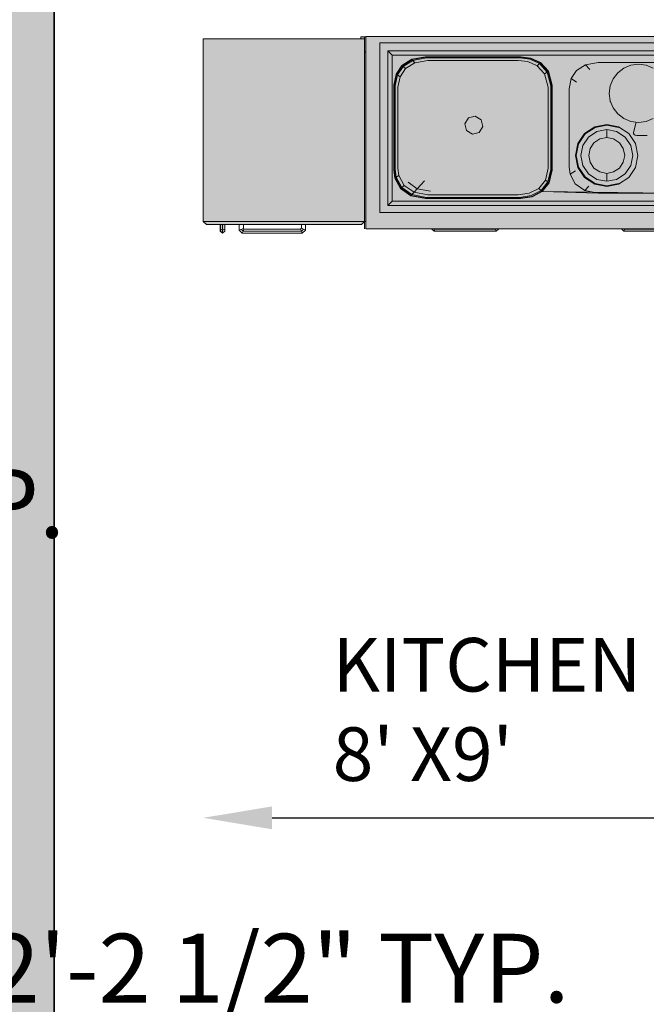
# Model space of a CAD drawing. Units: inches. Extents: x 2178 to 3409, y 1711 to 2279.
# Tile 5 of 8: x 2368 to 2423, y 2140 to 2226. Entities that reach past the tile are written whole.
import ezdxf

# ---------------------------------------------------------------- set-up
doc = ezdxf.new("R2010")
doc.units = ezdxf.units.IN
for name, color, linetype, lineweight in [('A-ANNO-DIMS', 2, 'Continuous', 18), ('A-AREA-IDEN', 7, 'Continuous', 18), ('A-FLOR-FIXT', 8, 'Continuous', 18), ('A-WALL', 7, 'Continuous', 35), ('A-WALL-PATT', 252, 'Continuous', 13)]:
    doc.layers.add(name, color=color, linetype=linetype, lineweight=lineweight)
doc.layers.add('hatch', color=254, linetype='Continuous')
doc.styles.get("Standard").update_dxf_attribs({"font": 'arial.ttf'})
doc.dimstyles.get("Standard").update_dxf_attribs({"dimtxt": 6, "dimasz": 6, "dimexe": 0.18, "dimexo": 0.0625, "dimgap": 0.09, "dimtad": 0, "dimtih": 1, "dimtoh": 1, "dimdec": 4, "dimzin": 0, "dimdsep": 46, "dimlunit": 4, "dimtxsty": 'Standard', "dimcen": 0.09, "dimse1": 1, "dimse2": 1, "dimadec": 0, "dimazin": 0, "dimtfac": 1, "dimtdec": 4, "dimtofl": 0, "dimtmove": 0, "dimatfit": 3, "dimfxl": 1, "dimtolj": 1, "dimtzin": 0, "dimarcsym": 0})

# ---------------------------------------------------------------- blocks, each defined once
blk = doc.blocks.new('kithen1')
at = {"layer": 'hatch'}
blk.add_hatch(color=256, dxfattribs=at).paths.add_polyline_path([(-2799.7, -8.3), (-2273.3, -8.3), (-2273.3, -1.7), (-2257.5, -1.7), (-2257.5, -1.1), (-1023.7, -1.1), (-1023.7, 0), (0, 0), (0, -0.3), (0.3, -0.3), (0.3, -1009.9), (-6.1, -1009.9), (-6.1, -2189.3), (-615.8, -2189.3), (-626.5, -2178.9), (-626.5, -1578.2), (-615.8, -1567.8), (-649.5, -1567.8), (-649.5, -1399.1), (-650.3, -1399.1), (-650.3, -1376.8), (-657.9, -1368.5), (-657.8, -1162.4), (-650.3, -1155.1), (-650.3, -1126.4), (-649.5, -1126.4), (-649.5, -1081.1), (-650.3, -1081.1), (-650.3, -1021.1), (-649.5, -1021.1), (-649.5, -959.1), (-651, -959.1), (-650.7, -903), (-653.5, -903), (-660.6, -895.5), (-660.5, -894.6), (-653.5, -887.1), (-651, -887.1), (-651, -638.7), (-651.2, -638.5), (-898.3, -638.5), (-898.3, -640.4), (-905.9, -647.4), (-906.8, -647.4), (-914.3, -640.4), (-914.3, -638.5), (-971.4, -638.5), (-971.4, -642.6), (-1016.2, -642.6), (-1016.2, -643.9), (-1023.8, -650.9), (-1024.7, -650.9), (-1032.2, -643.9), (-1032.2, -642.6), (-1179.7, -642.6), (-1188.8, -650.9), (-1395.6, -650.9), (-1403.7, -642.6), (-1813.5, -642.6), (-1822.6, -650.9), (-2029.4, -650.9), (-2037.5, -642.6), (-2257.5, -642.6), (-2257.5, -618.1), (-2261.3, -618.1), (-2271.7, -628.7), (-2458, -628.7), (-2727.7, -628.7), (-2727.7, -651.1), (-2735, -658.1), (-2735.9, -658), (-2743.2, -651.1), (-2743.2, -628.7), (-2789.4, -628.7), (-2799.7, -618.1)])
at = {"color": 0}
for p, q in [((-2261.3, -8.3), (-2799.7, -8.3)), ((-2799.7, -8.3), (-2799.7, -618.1)), ((-2273.3, -1.9), (-2273.9, -1.9)), ((-2273.9, -1.9), (-2273.9, -8.3)), ((-2261.3, -1.7), (-2273.3, -1.7)), ((-2273.3, -1.7), (-2273.3, -8.3)), ((-2261.3, -601.6), (-2261.3, -1.7)), ((-2261.3, -618.1), (-2261.3, -8.3)), ((-2261, -8.5), (-2261.3, -8.5)), ((-971.4, -1.1), (-2257.5, -1.1)), ((-2257.5, -1.1), (-2257.5, -642.6)), ((-1023.7, -22.5), (-2210.1, -22.5)), ((-2210.1, -22.5), (-2210.1, -589.1)), ((-2257.5, -51.5), (-2261.3, -51.5)), ((-2261.3, -51.5), (-2261.3, -536.3)), ((-2183.7, -48.8), (-1056.9, -48.9)), ((-2169.4, -62.7), (-2183.7, -48.8)), ((-2183.7, -48.8), (-2183.7, -565)), ((-2169.7, -550.2), (-2169.4, -62.7)), ((-1071, -63.6), (-2169.4, -62.7)), ((-2136.6, -97.6), (-2156.1, -126.2)), ((-2103.6, -76.6), (-2136.6, -97.6)), ((-2135.1, -98.9), (-2102.3, -78.1)), ((-2100.1, -80.6), (-2132.5, -101.2)), ((-2093.2, -88.3), (-2124.5, -108.2)), ((-2057.7, -68.5), (-2103.6, -76.6)), ((-2102.3, -78.1), (-2056.8, -70)), ((-2100.1, -80.6), (-2102.3, -78.1)), ((-2055, -72.6), (-2100.1, -80.6)), ((-2093.2, -88.3), (-2100.1, -80.6)), ((-2049.7, -80.6), (-2093.2, -88.3)), ((-1740.9, -68.5), (-2057.7, -68.5)), ((-2056.8, -70), (-1741.9, -70)), ((-1743.7, -72.6), (-2055, -72.6)), ((-1749, -80.6), (-2049.7, -80.6)), ((-1716.2, -84.8), (-1749, -80.6)), ((-1709.7, -76.9), (-1743.7, -72.6)), ((-1741.9, -70), (-1707.6, -74.4)), ((-1706.4, -72.9), (-1740.9, -68.5)), ((-1685.6, -98.8), (-1716.2, -84.8)), ((-1678, -91.5), (-1709.7, -76.9)), ((-1707.6, -74.4), (-1675.5, -89.1)), ((-1674.1, -87.7), (-1706.4, -72.9)), ((-1678, -91.5), (-1685.6, -98.8)), ((-1651.9, -119.5), (-1678, -91.5)), ((-1675.5, -89.1), (-1649.1, -117.4)), ((-1647.6, -116.2), (-1674.1, -87.7)), ((-1523.7, -95.6), (-1554, -114.9)), ((-1481.5, -88.1), (-1523.7, -95.6)), ((-1523.7, -95.6), (-1509.8, -111.1)), ((-1189.8, -88.1), (-1481.5, -88.1)), ((-1396, -106.6), (-1372.5, -96.9)), ((-1372.5, -96.9), (-1347.3, -93.6)), ((-1347.3, -93.6), (-1322, -96.9)), ((-1322, -96.9), (-1298.5, -106.6)), ((-2156.1, -126.2), (-2163.3, -163.2)), ((-2161.7, -164.1), (-2154.5, -127.3)), ((-2151.7, -129.3), (-2158.8, -165.7)), ((-2154.5, -127.3), (-2135.1, -98.9)), ((-2151.7, -129.3), (-2154.5, -127.3)), ((-2132.5, -101.2), (-2151.7, -129.3)), ((-2143, -135.3), (-2151.7, -129.3)), ((-2124.5, -108.2), (-2143, -135.3)), ((-2132.5, -101.2), (-2135.1, -98.9)), ((-2124.5, -108.2), (-2132.5, -101.2)), ((-1685.6, -98.8), (-1660.4, -125.8)), ((-1660.4, -125.8), (-1651.9, -119.5)), ((-1648.8, -170.4), (-1660.4, -125.8)), ((-1649.1, -117.4), (-1651.9, -119.5)), ((-1651.9, -119.5), (-1639.9, -165.7)), ((-1649.1, -117.4), (-1637, -164.1)), ((-1635.3, -163.2), (-1647.6, -116.2)), ((-1554, -114.9), (-1572, -141.2)), ((-1431.7, -142.2), (-1416.2, -122.1)), ((-1416.2, -122.1), (-1396, -106.6)), ((-2163.3, -163.2), (-2163.3, -447.5)), ((-2161.7, -446.6), (-2161.7, -164.1)), ((-2149.9, -170.5), (-2143, -135.3)), ((-1637, -164.1), (-1637, -446.6)), ((-1635.3, -447.4), (-1635.3, -163.2)), ((-1572, -141.2), (-1578.6, -175.3)), ((-1572, -141.2), (-1554.6, -153.3)), ((-1441.5, -165.7), (-1431.7, -142.2)), ((-2158.8, -165.7), (-2158.8, -445)), ((-2149.9, -440.2), (-2149.9, -170.5)), ((-1648.8, -440.2), (-1648.8, -170.4)), ((-1639.9, -165.7), (-1639.9, -445)), ((-1578.6, -175.3), (-1578.6, -437)), ((-1444.8, -190.8), (-1441.5, -165.7)), ((-1441.5, -216), (-1444.8, -190.8)), ((-1442, -212), (-1442.1, -213.6)), ((-1442.1, -213.6), (-1441.9, -216.3)), ((-1441.9, -216.3), (-1441.5, -218.2)), ((-1431.7, -239.4), (-1441.5, -216)), ((-1441.5, -218.2), (-1440.8, -218.9)), ((-1440.8, -218.9), (-1440.3, -218.9)), ((-1416.2, -259.6), (-1431.7, -239.4)), ((-1396, -275), (-1416.2, -259.6)), ((-1914.6, -272.1), (-1926.9, -292)), ((-1926.9, -292), (-1921.4, -314.8)), ((-1891.8, -266.6), (-1914.6, -272.1)), ((-1871.8, -278.8), (-1891.8, -266.6)), ((-1866.3, -301.6), (-1871.8, -278.8)), ((-1493.1, -302.1), (-1453.2, -294.2)), ((-1453.2, -294.3), (-1493.1, -302.2)), ((-1453.2, -294.2), (-1413.4, -302.1)), ((-1413.4, -302.2), (-1453.2, -294.3)), ((-1453.2, -294.3), (-1453.2, -296.5)), ((-1372.5, -284.8), (-1396, -275)), ((-1347.3, -288.1), (-1372.5, -284.8)), ((-1364, -321.4), (-1354.5, -287.1)), ((-1322, -284.8), (-1347.3, -288.1)), ((-1298.5, -275), (-1322, -284.8)), ((-1921.4, -314.8), (-1901.4, -327)), ((-1901.4, -327), (-1878.5, -321.5)), ((-1878.5, -321.5), (-1866.3, -301.6)), ((-1526.8, -324.6), (-1549.4, -358.3)), ((-1549.4, -358.3), (-1526.8, -324.6)), ((-1525.2, -326.2), (-1547.3, -359.2)), ((-1526.8, -324.6), (-1493.1, -302.1)), ((-1493.1, -302.2), (-1526.8, -324.6)), ((-1492.2, -304.2), (-1525.2, -326.2)), ((-1486.4, -318.2), (-1514.5, -337)), ((-1453.2, -296.5), (-1492.2, -304.2)), ((-1453.2, -311.7), (-1486.4, -318.2)), ((-1453.2, -296.5), (-1414.2, -304.2)), ((-1453.2, -311.7), (-1420.1, -318.2)), ((-1453.2, -338.2), (-1453.2, -311.7)), ((-1420.1, -318.2), (-1392, -337)), ((-1413.4, -302.1), (-1379.6, -324.6)), ((-1379.6, -324.6), (-1413.4, -302.2)), ((-1379.6, -324.6), (-1357, -358.3)), ((-1357, -358.3), (-1379.6, -324.6)), ((-1363.6, -324.3), (-1364, -321.4)), ((-1361.6, -328), (-1363.6, -324.3)), ((-1357.9, -330.6), (-1361.6, -328)), ((-1549.4, -358.3), (-1557.3, -398)), ((-1557.3, -398), (-1549.4, -358.3)), ((-1547.3, -359.2), (-1555.1, -398)), ((-1514.5, -337), (-1533.3, -365)), ((-1508.7, -375.1), (-1495.7, -355.7)), ((-1495.7, -355.7), (-1476.2, -342.8)), ((-1476.2, -342.8), (-1453.2, -338.2)), ((-1430.3, -342.8), (-1453.2, -338.2)), ((-1410.8, -355.7), (-1430.3, -342.8)), ((-1397.8, -375.1), (-1410.8, -355.7)), ((-1392, -337), (-1373.2, -365)), ((-1352.7, -331.6), (-1357.9, -330.6)), ((-1357, -358.3), (-1349.1, -398)), ((-1349.1, -398), (-1357, -358.3)), ((-1318.5, -331.6), (-1352.7, -331.6)), ((-1533.3, -365), (-1539.9, -398)), ((-1513.2, -398), (-1508.7, -375.1)), ((-1393.2, -398), (-1397.8, -375.1)), ((-1373.2, -365), (-1366.6, -398)), ((-1557.3, -398), (-1549.4, -437.8)), ((-1549.4, -437.8), (-1557.3, -398)), ((-1555.1, -398), (-1547.3, -436.9)), ((-1539.9, -398), (-1533.3, -431.1)), ((-1508.7, -420.9), (-1513.2, -398)), ((-1495.7, -440.4), (-1508.7, -420.9)), ((-1410.8, -440.4), (-1397.8, -420.9)), ((-1397.8, -420.9), (-1393.2, -398)), ((-1366.6, -398), (-1373.2, -431.1)), ((-1349.1, -398), (-1357, -437.8)), ((-1357, -437.8), (-1349.1, -398)), ((-2163.3, -447.5), (-2159.9, -473.6)), ((-2158.2, -472.6), (-2161.7, -446.6)), ((-2158.8, -445), (-2155.4, -470.7)), ((-2146.6, -465), (-2149.9, -440.2)), ((-1658, -480.4), (-1648.8, -440.2)), ((-1639.9, -445), (-1649.4, -486.6)), ((-1637, -446.6), (-1646.6, -488.6)), ((-1645, -489.8), (-1635.3, -447.4)), ((-1578.6, -437), (-1575.5, -461.1)), ((-1575.5, -461.1), (-1557.8, -449.7)), ((-1549.4, -437.8), (-1526.8, -471.4)), ((-1526.8, -471.4), (-1549.4, -437.8)), ((-1547.3, -436.9), (-1525.2, -469.8)), ((-1533.3, -431.1), (-1514.5, -459.1)), ((-1514.5, -459.1), (-1486.4, -477.9)), ((-1476.2, -453.3), (-1495.7, -440.4)), ((-1453.2, -457.9), (-1476.2, -453.3)), ((-1453.2, -457.9), (-1430.3, -453.3)), ((-1453.2, -484.4), (-1453.2, -457.9)), ((-1430.3, -453.3), (-1410.8, -440.4)), ((-1392, -459.1), (-1420.1, -477.9)), ((-1373.2, -431.1), (-1392, -459.1)), ((-1357, -437.8), (-1379.6, -471.4)), ((-1379.6, -471.4), (-1357, -437.8)), ((-2159.9, -473.6), (-2141.1, -508.3)), ((-2139.6, -507.1), (-2158.2, -472.6)), ((-2155.4, -470.7), (-2146.6, -465)), ((-2137, -504.8), (-2155.4, -470.7)), ((-2146.6, -465), (-2128.8, -498)), ((-2085.5, -509.3), (-2116.3, -487.4)), ((-2060.9, -482.3), (-2085.5, -509.3)), ((-1680.2, -507.9), (-1658, -480.4)), ((-1649.4, -486.6), (-1672.5, -515.1)), ((-1646.6, -488.6), (-1669.9, -517.4)), ((-1668.5, -518.8), (-1645, -489.8)), ((-1649.4, -486.6), (-1658, -480.4)), ((-1646.6, -488.6), (-1649.4, -486.6)), ((-1575.5, -461.1), (-1558.2, -493)), ((-1558.2, -493), (-1526.7, -515.5)), ((-1493.1, -493.9), (-1526.8, -471.4)), ((-1526.8, -471.4), (-1493.1, -493.9)), ((-1525.2, -469.8), (-1492.2, -491.9)), ((-1492.2, -491.9), (-1453.2, -499.6)), ((-1486.4, -477.9), (-1453.2, -484.4)), ((-1420.1, -477.9), (-1453.2, -484.4)), ((-1453.2, -499.6), (-1414.2, -491.9)), ((-1379.6, -471.4), (-1413.4, -493.9)), ((-1413.4, -493.9), (-1379.6, -471.4)), ((-2141.1, -508.3), (-2106.9, -532.7)), ((-2137, -504.8), (-2139.6, -507.1)), ((-2105.6, -531.3), (-2139.6, -507.1)), ((-2128.8, -498), (-2137, -504.8)), ((-2103.3, -528.8), (-2137, -504.8)), ((-2128.8, -498), (-2096.3, -521.1)), ((-2096.3, -521.1), (-2103.3, -528.8)), ((-2096.3, -521.1), (-2085.5, -509.3)), ((-2049.7, -530.1), (-2096.3, -521.1)), ((-2085.5, -509.3), (-2041.5, -517.8)), ((-1711.5, -524.5), (-1749, -530.1)), ((-1680.2, -507.9), (-1711.5, -524.5)), ((-1672.5, -515.1), (-1704.9, -532.3)), ((-1702.7, -534.9), (-1669.9, -517.4)), ((-1668.5, -518.8), (-1701.5, -536.3)), ((-1672.5, -515.1), (-1680.2, -507.9)), ((-1669.9, -517.4), (-1672.5, -515.1)), ((-1189.8, -524.2), (-1668.5, -518.8)), ((-1481.5, -524.2), (-1668.5, -518.8)), ((-1526.7, -515.5), (-1512.6, -500.1)), ((-1526.7, -515.5), (-1481.5, -524.2)), ((-1453.2, -501.8), (-1493.1, -493.9)), ((-1493.1, -493.9), (-1453.2, -501.8)), ((-1189.8, -524.2), (-1481.5, -524.2)), ((-1413.4, -493.9), (-1453.2, -501.8)), ((-1453.2, -501.8), (-1413.4, -493.9)), ((-1453.2, -499.6), (-1453.2, -501.8)), ((-2257.5, -535.3), (-2257.9, -535.3)), ((-2183.7, -565), (-2169.7, -550.2)), ((-1793.1, -550.2), (-2169.7, -550.2)), ((-2106.9, -532.7), (-2057.7, -542.2)), ((-2103.3, -528.8), (-2105.6, -531.3)), ((-2056.8, -540.7), (-2105.6, -531.3)), ((-2055, -538.1), (-2103.3, -528.8)), ((-2057.7, -542.2), (-2056.8, -540.7)), ((-1783.5, -542.2), (-2057.7, -542.2)), ((-1781.7, -540.7), (-2056.8, -540.7)), ((-1778.6, -538.1), (-2055, -538.1)), ((-1749, -530.1), (-2049.7, -530.1)), ((-1749, -530.1), (-1797.1, -530.1)), ((-1743.7, -538.1), (-1797.1, -538.1)), ((-1741.9, -540.7), (-1797.1, -540.7)), ((-1740.9, -542.2), (-1797.1, -542.2)), ((-1071, -550.2), (-1797.1, -550.2)), ((-1704.9, -532.3), (-1743.7, -538.1)), ((-1741.9, -540.7), (-1702.7, -534.9)), ((-1740.9, -542.2), (-1741.9, -540.7)), ((-1701.5, -536.3), (-1740.9, -542.2)), ((-2210.1, -589.1), (-1789.4, -589.1)), ((-1797.1, -565), (-2183.7, -565)), ((-1056.9, -565), (-1797.1, -565)), ((-1797.1, -589.1), (-1023.7, -589.1)), ((-2799.7, -618.1), (-2261.3, -618.1)), ((-2789.4, -628.7), (-2799.7, -618.1)), ((-2261.3, -618.1), (-2271.7, -628.7)), ((-2261, -596.4), (-2261.3, -596.4)), ((-2261.3, -626.3), (-2261.3, -601.6)), ((-2271.7, -628.7), (-2789.4, -628.7)), ((-2743.2, -628.7), (-2743.2, -644.8)), ((-2743.2, -644.8), (-2742.3, -644.5)), ((-2743.2, -651.1), (-2743.2, -644.8)), ((-2742.3, -650.3), (-2743.2, -651.1)), ((-2742.3, -651.1), (-2743.2, -651.1)), ((-2743.2, -651.1), (-2735.9, -658)), ((-2742.3, -628.7), (-2742.3, -644.4)), ((-2742.3, -644.4), (-2734.9, -647.4)), ((-2742.3, -644.4), (-2742.3, -651.1)), ((-2735, -658.1), (-2742.3, -651.1)), ((-2734.9, -647.4), (-2735, -658.1)), ((-2735, -658.1), (-2727.7, -651.1)), ((-2734.9, -647.4), (-2734.9, -628.7)), ((-2727.7, -644.4), (-2734.9, -647.4)), ((-2727.7, -628.7), (-2727.7, -644.4)), ((-2727.7, -651.1), (-2727.7, -644.4)), ((-2679.7, -628.7), (-2679.4, -647.7)), ((-2679.4, -647.7), (-2665.9, -642)), ((-2669.5, -658), (-2679.4, -647.7)), ((-2666.7, -651.1), (-2672.6, -644.8)), ((-2666.7, -651.1), (-2669.5, -658)), ((-2663.9, -644.2), (-2666.7, -651.1)), ((-2472.3, -651.1), (-2666.7, -651.1)), ((-2665.6, -628.7), (-2665.9, -642)), ((-2665.9, -642), (-2663.9, -644.2)), ((-2663.9, -644.2), (-2474.9, -644.1)), ((-2474.9, -644.1), (-2471.7, -641.3)), ((-2474.9, -644.1), (-2472.3, -651.1)), ((-2472.3, -651.1), (-2465, -644.4)), ((-2469.7, -658.1), (-2472.3, -651.1)), ((-2471.7, -641.3), (-2472, -628.7)), ((-2458.4, -647.4), (-2471.7, -641.3)), ((-2458.4, -647.4), (-2469.7, -658.1)), ((-2458, -628.7), (-2458.4, -647.4)), ((-2261.3, -643.6), (-2261.3, -626.3)), ((-2257.5, -642.6), (-1797.1, -642.6)), ((-2037.5, -642.6), (-2029.4, -650.9)), ((-2029.4, -650.9), (-2026.5, -643.9)), ((-2029.4, -650.9), (-1828.9, -650.9)), ((-2026.5, -643.9), (-2027.8, -642.6)), ((-2025.9, -642.6), (-2026.5, -643.9)), ((-2026.5, -643.9), (-1828.9, -643.9)), ((-1825.3, -643.9), (-1828.9, -643.9)), ((-1822.6, -650.9), (-1828.9, -650.9)), ((-1825.8, -642.6), (-1825.3, -643.9)), ((-1825.3, -643.9), (-1823.8, -642.6)), ((-1822.6, -650.9), (-1825.3, -643.9)), ((-1813.5, -642.6), (-1822.6, -650.9)), ((-971.4, -642.6), (-1797.1, -642.6)), ((-1395.6, -650.9), (-1403.7, -642.6)), ((-1392.7, -643.9), (-1395.6, -650.9)), ((-1395.6, -650.9), (-1188.8, -650.9)), ((-1394, -642.6), (-1392.7, -643.9)), ((-1392.7, -643.9), (-1392.1, -642.6)), ((-1191.5, -643.9), (-1392.7, -643.9)), ((-2735.9, -658), (-2735, -658.1)), ((-2669.5, -658), (-2469.7, -658.1))]:
    blk.add_line(p, q, dxfattribs=at)
for points in [[(-2799.7, -8.3), (-2273.3, -8.3), (-2273.3, -1.7), (-2257.5, -1.7), (-2257.5, -1.1), (-1023.7, -1.1)], [(-1188.8, -650.9), (-1395.6, -650.9), (-1403.7, -642.6), (-1813.5, -642.6), (-1822.6, -650.9), (-2029.4, -650.9), (-2037.5, -642.6), (-2257.5, -642.6), (-2257.5, -618.1), (-2261.3, -618.1), (-2271.7, -628.7), (-2458, -628.7), (-2727.7, -628.7), (-2727.7, -651.1), (-2735, -658.1), (-2735.9, -658), (-2743.2, -651.1), (-2743.2, -628.7), (-2789.4, -628.7), (-2799.7, -618.1), (-2799.7, -8.3)]]:
    blk.add_lwpolyline(points)
blk = doc.blocks.new('*D37')
at = {"layer": 'A-ANNO-DIMS', "color": 0, "lineweight": -2, "transparency": 16777216}
for p, q in [((2323.494, 2208.611), (2323.494, 2186.605)), ((2323.494, 2158.209), (2323.494, 2180.216))]:
    blk.add_line(p, q, dxfattribs=at)
at = {"layer": 'A-ANNO-DIMS', "color": 0, "transparency": 16777216}
for points in [[(2322.494, 2208.611), (2324.494, 2208.611), (2323.494, 2214.611)], [(2322.494, 2158.209), (2324.494, 2158.209), (2323.494, 2152.209)]]:
    blk.add_solid(points, dxfattribs=at)
at = {"layer": 'Defpoints', "color": 0, "transparency": 16777216}
for p in [(2332.854, 2214.611), (2323.494, 2152.209), (2332.854, 2152.209)]:
    blk.add_point(p, dxfattribs=at)
at = {"layer": 'A-ANNO-DIMS', "color": 0, "transparency": 16777216, "insert": (2323.494, 2183.41), "char_height": 6, "attachment_point": 5}
blk.add_mtext('\\A1;WARDROBE 5\'-2 1/2" TYP.', dxfattribs=at)
blk = doc.blocks.new('*D38')
at = {"layer": 'A-ANNO-DIMS', "color": 0, "lineweight": -2, "transparency": 16777216}
for p, q in [((2338.854, 2142.849), (2353.232, 2142.849)), ((2359.232, 2142.849), (2365.232, 2142.849))]:
    blk.add_line(p, q, dxfattribs=at)
at = {"layer": 'A-ANNO-DIMS', "color": 0, "transparency": 16777216}
for points in [[(2338.854, 2143.849), (2338.854, 2141.849), (2332.854, 2142.849)], [(2353.232, 2143.849), (2353.232, 2141.849), (2359.232, 2142.849)]]:
    blk.add_solid(points, dxfattribs=at)
at = {"layer": 'Defpoints', "color": 0, "transparency": 16777216}
for p in [(2332.854, 2152.209), (2359.232, 2152.209), (2359.232, 2142.849)]:
    blk.add_point(p, dxfattribs=at)
at = {"layer": 'A-ANNO-DIMS', "color": 0, "transparency": 16777216, "insert": (2390.65, 2142.849), "char_height": 6, "attachment_point": 5}
blk.add_mtext('\\A1;2\'-2 1/2" TYP.', dxfattribs=at)
blk = doc.blocks.new('*D47')
at = {"layer": 'A-ANNO-DIMS', "color": 0, "lineweight": -2, "transparency": 16777216}
for p, q in [((2291.224, 2232.643), (2315.224, 2232.643)), ((2321.224, 2232.643), (2327.224, 2232.643))]:
    blk.add_line(p, q, dxfattribs=at)
at = {"layer": 'A-ANNO-DIMS', "color": 0, "transparency": 16777216}
for points in [[(2291.224, 2233.643), (2291.224, 2231.643), (2285.224, 2232.643)], [(2315.224, 2233.643), (2315.224, 2231.643), (2321.224, 2232.643)]]:
    blk.add_solid(points, dxfattribs=at)
at = {"layer": 'Defpoints', "color": 0, "transparency": 16777216}
for p in [(2285.224, 2238.043), (2321.224, 2238.043), (2321.224, 2232.643)]:
    blk.add_point(p, dxfattribs=at)
at = {"layer": 'A-ANNO-DIMS', "color": 0, "transparency": 16777216, "insert": (2365.276, 2232.643), "char_height": 6, "attachment_point": 5}
blk.add_mtext('\\A1;WINDOW 3\'-0" TYP.', dxfattribs=at)
blk = doc.blocks.new('*D57')
at = {"layer": 'A-ANNO-DIMS', "color": 0, "lineweight": -2, "transparency": 16777216}
for p, q in [((2390.072, 2155.967), (2451.379, 2155.967)), ((2457.379, 2155.967), (2463.379, 2155.967))]:
    blk.add_line(p, q, dxfattribs=at)
at = {"layer": 'A-ANNO-DIMS', "color": 0, "transparency": 16777216}
for points in [[(2390.072, 2156.967), (2390.072, 2154.967), (2384.072, 2155.967)], [(2451.379, 2156.967), (2451.379, 2154.967), (2457.379, 2155.967)]]:
    blk.add_solid(points, dxfattribs=at)
at = {"layer": 'Defpoints', "color": 0, "transparency": 16777216}
for p in [(2384.072, 2166.963), (2457.379, 2166.963), (2457.379, 2155.967)]:
    blk.add_point(p, dxfattribs=at)
at = {"layer": 'A-ANNO-DIMS', "color": 0, "transparency": 16777216, "insert": (2500.286, 2155.967), "char_height": 6, "attachment_point": 5}
blk.add_mtext('\\A1;COUNTER 6\'-1 1/2"', dxfattribs=at)
blk = doc.blocks.new('*D71')
at = {"layer": 'A-ANNO-DIMS', "color": 0, "lineweight": -2, "transparency": 16777216}
for p, q in [((2381.625685, 2275.292563), (2375.625685, 2275.292563)), ((2410.582731, 2275.292563), (2416.582731, 2275.292563))]:
    blk.add_line(p, q, dxfattribs=at)
at = {"layer": 'A-ANNO-DIMS', "color": 0, "transparency": 16777216}
for points in [[(2381.625685, 2276.292563), (2381.625685, 2274.292563), (2387.625685, 2275.292563)], [(2410.582731, 2276.292563), (2410.582731, 2274.292563), (2404.582731, 2275.292563)]]:
    blk.add_solid(points, dxfattribs=at)
at = {"layer": 'Defpoints', "color": 0, "transparency": 16777216}
for p in [(2404.582731, 2275.292563), (2387.625685, 1942.827852), (2404.582731, 1942.827852)]:
    blk.add_point(p, dxfattribs=at)
at = {"layer": 'A-ANNO-DIMS', "color": 0, "transparency": 16777216, "insert": (2396.104208, 2275.292563), "char_height": 6, "attachment_point": 5}
blk.add_mtext('\\A1;1\'-5"', dxfattribs=at)
blk = doc.blocks.new('*D73')
at = {"layer": 'A-ANNO-DIMS', "color": 0, "lineweight": -2, "transparency": 16777216}
for p, q in [((2387.374, 2275.293), (2388.322, 2275.293)), ((2405.502, 2275.293), (2404.554, 2275.293))]:
    blk.add_line(p, q, dxfattribs=at)
at = {"layer": 'A-ANNO-DIMS', "color": 0, "transparency": 16777216}
for points in [[(2387.374, 2276.293), (2387.374, 2274.293), (2381.374, 2275.293)], [(2405.502, 2276.293), (2405.502, 2274.293), (2411.502, 2275.293)]]:
    blk.add_solid(points, dxfattribs=at)
at = {"layer": 'Defpoints', "color": 0, "transparency": 16777216}
for p in [(2411.502, 2275.293), (2381.374, 1966.488), (2411.502, 1966.488)]:
    blk.add_point(p, dxfattribs=at)
at = {"layer": 'A-ANNO-DIMS', "color": 0, "transparency": 16777216, "insert": (2396.438, 2275.293), "char_height": 6, "attachment_point": 5}
blk.add_mtext('\\A1;2\'-6"', dxfattribs=at)

msp = doc.modelspace()

# ---------------------------------------------------------------- hatches: boundary and pattern name
at = {"layer": 'A-WALL-PATT'}
h = msp.add_hatch(color=256, dxfattribs=at)
h.dxf.hatch_style = 1
h.paths.add_polyline_path([(2233.06485, 1992.04256), (2317.06485, 1992.04256), (2317.06485, 1998.04256), (2317.06485, 2006.75072), (2311.06485, 2006.75072), (2311.06485, 1998.04256), (2233.06485, 1998.04256), (2233.06485, 2009.64251), (2224.06485, 2009.64251), (2224.06485, 1863.04256), (2233.06485, 1863.04256), (2278.65041, 1863.04256), (2278.65041, 1872.04256), (2233.06485, 1872.04256)])
h.paths.add_polyline_path([(2359.06485, 1992.04256), (2359.06485, 1998.04256), (2353.06485, 1998.04256), (2353.06485, 1962.04256), (2353.06485, 1872.04256), (2314.65041, 1872.04256), (2314.65041, 1863.04256), (2359.06485, 1863.04256), (2359.06485, 1872.04256)])
h.paths.add_polyline_path([(2401.06485, 1890.04256), (2371.06485, 1890.04256), (2359.06485, 1890.04256), (2359.06485, 1884.04256), (2371.06485, 1884.04256), (2377.06485, 1884.04256), (2401.06485, 1884.04256)])
h.paths.add_polyline_path([(2353.06485, 1802.77269), (2359.06485, 1802.77269), (2359.06485, 1808.77269), (2356.83755, 1808.77269), (2353.06485, 1808.77269), (2347.91295, 1808.77269), (2347.91295, 1802.77269), (2347.91295, 1749.04256), (2342.02347, 1749.04256), (2342.02347, 1743.04256), (2353.06485, 1743.04256)])
h.paths.add_polyline_path([(2476.06485, 2247.04256), (2442.91353, 2247.04256), (2442.91353, 2238.04256), (2467.06485, 2238.04256), (2467.06485, 2041.93675), (2476.06485, 2041.93675)])
h.paths.add_polyline_path([(2467.06485, 2106.04256), (2406.56133, 2106.04256, -0.04188649), (2407.06485, 2100.04256), (2467.06485, 2100.04256)])
h.paths.add_polyline_path([(2406.91353, 2247.04256), (2321.22384, 2247.04256), (2321.22384, 2238.04256), (2365.06485, 2238.04256), (2365.06485, 2106.04256), (2365.06485, 2100.04256), (2371.06485, 2100.04256), (2371.06485, 2136.04256), (2371.06485, 2238.04256), (2406.91353, 2238.04256)])
h.paths.add_polyline_path([(2285.22384, 2247.04256), (2224.06485, 2247.04256), (2224.06485, 2087.1459), (2233.06485, 2087.1459), (2233.06485, 2100.04256), (2329.06485, 2100.04256, -0.04188649), (2329.56837, 2106.04256), (2233.06485, 2106.04256), (2233.06485, 2238.04256), (2285.22384, 2238.04256)])
h.paths.add_polyline_path([(2317.06485, 2052.04256), (2317.06485, 2061.5418), (2311.06485, 2061.5418), (2311.06485, 2052.04256), (2233.06485, 2052.04256), (2233.06485, 2063.1459), (2224.06485, 2063.1459), (2224.06485, 2033.64251), (2233.06485, 2033.64251), (2233.06485, 2046.04256), (2311.06485, 2046.04256), (2311.06485, 2036.1446, -0.05038204), (2317.06485, 2036.75072), (2317.06485, 2046.04256)])

# ---------------------------------------------------------------- linework, layer by layer
at = {"layer": 'A-WALL'}
msp.add_line((2371.06485, 2238.04256), (2371.06485, 2106.04256), dxfattribs=at)

# ---------------------------------------------------------------- block references
at = {"layer": 'A-FLOR-FIXT', "xscale": 0.0261336107367163, "yscale": 0.0261336107367163, "zscale": 0.0261336107367163}
msp.add_blockref('kithen1', (2457.23906, 2224.17699), dxfattribs=at)

# ---------------------------------------------------------------- texts
at = {"layer": 'A-AREA-IDEN', "insert": (2395.36185, 2171.66551), "char_height": 4.679699, "attachment_point": 1}
msp.add_mtext_dynamic_manual_height_columns("KITCHEN \\P8' X9'", width=123.0595467, gutter_width=23.3985, heights=[41.64659], dxfattribs=at)

# ---------------------------------------------------------------- dimensions: what is measured, and where the dimension line sits
at = {"layer": 'A-ANNO-DIMS'}
for base, p1, p2, picture, middle in [((2404.58273, 2275.29256), (2387.62568, 1942.82785), (2404.58273, 1942.82785), '*D71', (2396.10421, 2275.29256)), ((2411.50157, 2275.29256), (2381.37394, 1966.48789), (2411.50157, 1966.48789), '*D73', (2396.43775, 2275.29256))]:
    dim = msp.add_linear_dim(base=base, p1=p1, p2=p2, dimstyle='Standard', override={"dimdec": 1, "dimlfac": 1, "dimrnd": 0, "dimzin": 1, "dimdsep": 46, "dimlunit": 4, "dimfrac": 2}, dxfattribs=at)
    dim.commit()
    dim.dimension.update_dxf_attribs({"geometry": picture, "text_midpoint": middle})
for base, p1, p2, text, picture, middle in [((2321.22384, 2232.64256), (2285.22384, 2238.04256), (2321.22384, 2238.04256), 'WINDOW <> TYP.', '*D47', (2365.27632, 2232.64256)), ((2457.37908, 2155.96728), (2384.07233, 2166.96329), (2457.37908, 2166.96329), 'COUNTER <>', '*D57', (2500.28559, 2155.96728)), ((2359.23207, 2142.84918), (2332.85429, 2152.20941), (2359.23207, 2152.20941), '<> TYP.', '*D38', (2390.65017, 2142.84918))]:
    dim = msp.add_linear_dim(base=base, p1=p1, p2=p2, text=text, dimstyle='Standard', override={"dimdec": 1, "dimlfac": 1, "dimrnd": 0, "dimzin": 1, "dimdsep": 46, "dimlunit": 4, "dimfrac": 2}, dxfattribs=at)
    dim.commit()
    dim.dimension.update_dxf_attribs({"geometry": picture, "text_midpoint": middle})
dim = msp.add_linear_dim(base=(2323.49406, 2152.20941), p1=(2332.85429, 2214.61099), p2=(2332.85429, 2152.20941), angle=270, text='WARDROBE <> TYP.', dimstyle='Standard', override={"dimdec": 1, "dimlfac": 1, "dimrnd": 0, "dimzin": 1, "dimdsep": 46, "dimlunit": 4, "dimfrac": 2}, dxfattribs=at)
dim.commit()
dim.dimension.update_dxf_attribs({"geometry": '*D37', "text_midpoint": (2323.49406, 2183.4102)})

doc.saveas('drawing.dxf')
